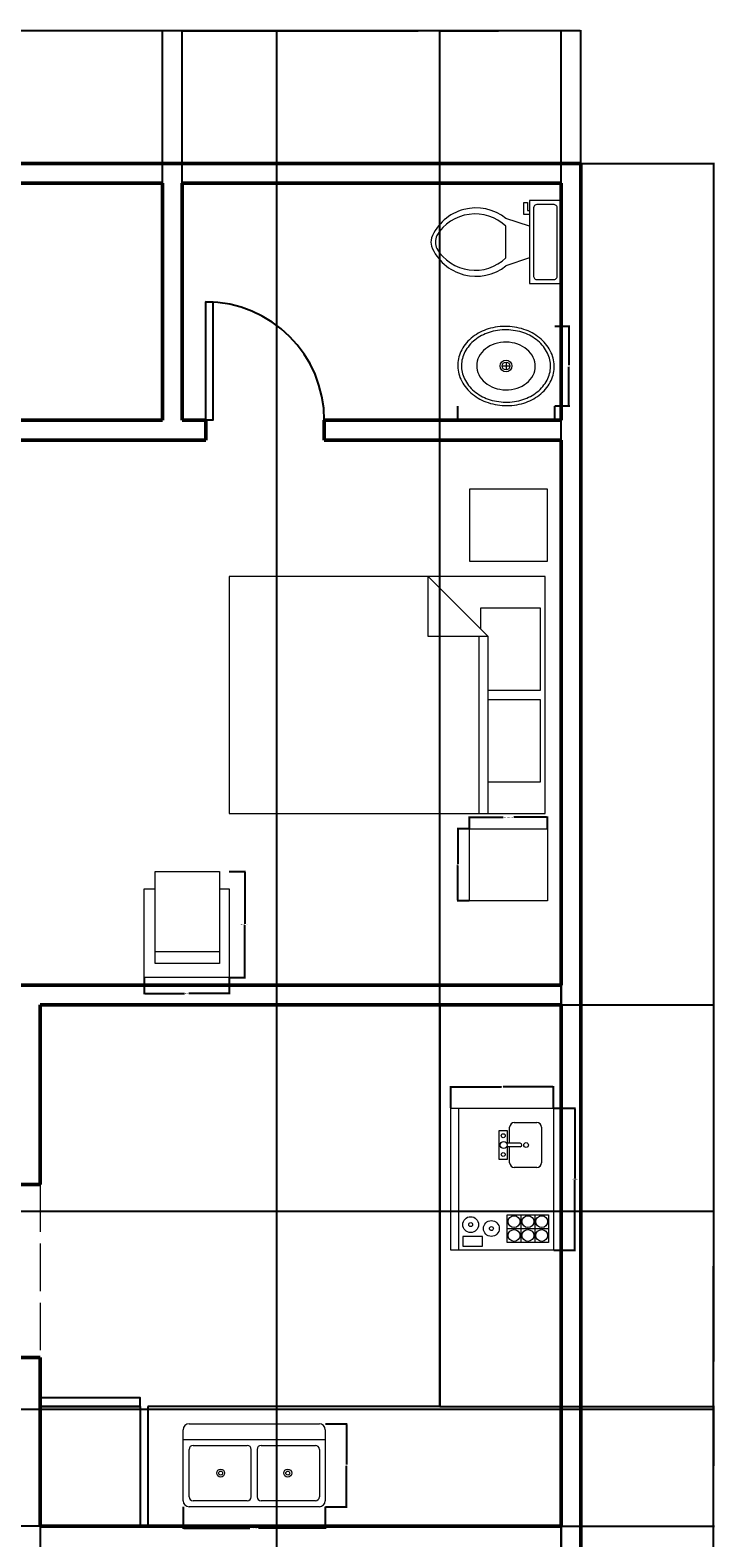
# Model space of a CAD drawing. Units: inches. Extents: x 115999 to 116502, y 188991 to 189729.
# Tile 5 of 5: x 116329 to 116502, y 189347 to 189729. Entities that reach past the tile are written whole.
import ezdxf

# ---------------------------------------------------------------- set-up
doc = ezdxf.new("R2010")
doc.units = ezdxf.units.IN
doc.linetypes.add('ACAD_ISO02W100', pattern=[15, 12, -3])
for name, color, linetype, lineweight in [('A-ANNO-DIMS', 2, 'Continuous', 18), ('A-DOOR', 4, 'Continuous', 25), ('A-FLOR-CASE', 9, 'Continuous', 25), ('A-FLOR-FIXT', 9, 'Continuous', 20), ('A-FURN', 8, 'Continuous', 18), ('A-WALL', 7, 'Continuous', 50), ('A-WALL-OVHD', 7, 'ACAD_ISO02W100', 18)]:
    doc.layers.add(name, color=color, linetype=linetype, lineweight=lineweight)
doc.styles.get("Standard").update_dxf_attribs({"font": 'arial.ttf'})
doc.dimstyles.get("Standard").update_dxf_attribs({"dimtxt": 0.18, "dimasz": 0.18, "dimexe": 0.18, "dimexo": 0.0625, "dimgap": 0.09, "dimtad": 0, "dimtih": 1, "dimtoh": 1, "dimdec": 4, "dimzin": 0, "dimdsep": 46, "dimtxsty": 'Standard', "dimcen": 0.09, "dimadec": 0, "dimazin": 0, "dimtfac": 1, "dimtdec": 4, "dimtofl": 0, "dimtmove": 0, "dimatfit": 3, "dimfxl": 1, "dimtolj": 1, "dimtzin": 0, "dimarcsym": 0})

# ---------------------------------------------------------------- blocks, each defined once
blk = doc.blocks.new('*U3')
for p, q in [((0, 0), (0, -5)), ((30, 0), (30, -5))]:
    blk.add_line(p, q)
blk.add_lwpolyline([(0, 0), (0, 30), (1.75, 30), (1.75, 0)], close=True)
blk.add_arc((0, 0), 30, 0, 90)
blk = doc.blocks.new('Wet Bar')
for p, q in [((0, 0), (36, 0)), ((0, -26), (0, 0)), ((36, 0), (36, -26)), ((0, -2), (36, -2)), ((3.5, -3), (1, -3)), ((1, -3), (1, -8)), ((3.5, -8), (3.5, -3)), ((1, -8), (3.5, -8)), ((2, -14.25), (9, -14.25)), ((2, -24.75), (2, -14.25)), ((5.5, -14.25), (5.5, -24.75)), ((9, -14.25), (9, -24.75)), ((26.2, -17.55), (26.2, -14.1284)), ((27.1001, -17.55), (27.1001, -14.1284)), ((2, -17.75), (9, -17.75)), ((9, -21.25), (2, -21.25)), ((36, -26), (0, -26)), ((9, -24.75), (2, -24.75))]:
    blk.add_line(p, q)
for points in [[(22.15, -14.85), (26.2, -14.85)], [(26.2, -14.25), (22.95, -14.25), (22.95, -12.2), (26.75, -12.2)], [(26.7487, -12.2), (30.3501, -12.2), (30.3501, -14.25), (27.1001, -14.25)], [(27.1001, -14.85), (31.15, -14.85)], [(20.95, -21.75), (20.95, -16.05)], [(32.3501, -16.05), (32.3501, -21.75)], [(31.15, -22.95), (22.15, -22.95)]]:
    blk.add_lwpolyline(points)
for centre, radius in [((6.5, -5), 2), ((6.5, -5), 0.5), ((5.5, -10.25), 2), ((5.5, -10.25), 0.5), ((3.75, -16), 1.5), ((7.25, -16), 1.5), ((24.25, -13.25), 0.5), ((26.65, -13.35), 0.9), ((29, -13.25), 0.5), ((3.75, -19.5), 1.5), ((7.25, -19.5), 1.5), ((26.65, -19.05), 0.6), ((3.75, -23), 1.5), ((7.25, -23), 1.5)]:
    blk.add_circle(centre, radius)
for centre, radius, start, end in [((22.2251, -16.125), 1.2772, 93.36646, 176.6335), ((31.075, -16.125), 1.2772, 3.366461, 86.63354), ((26.65, -17.55), 0.45, 180, 0), ((22.2251, -21.675), 1.2772, 183.3665, 266.6335), ((31.075, -21.675), 1.2772, 273.3665, 356.6335)]:
    blk.add_arc(centre, radius, start, end)
blk = doc.blocks.new('Sink-double - 36 in top')
for p, q in [((-18, -4), (18, -4)), ((-0.75, -18.5), (-0.75, -6.5)), ((0.75, -6.5), (0.75, -18.5))]:
    blk.add_line(p, q)
for points in [[(-16.5, 0), (16.5, 0)], [(-18, -19.5), (-18, -1.5)], [(18, -1.5), (18, -19.5)], [(-16.5, -18.5), (-16.5, -6.5)], [(-15.5, -5.5), (-1.75, -5.5)], [(1.75, -5.5), (15.5, -5.5)], [(16.5, -6.5), (16.5, -18.5)], [(16.5, -21), (-16.5, -21)], [(-1.75, -19.5), (-15.5, -19.5)], [(15.5, -19.5), (1.75, -19.5)]]:
    blk.add_lwpolyline(points)
for centre, radius in [((-8.5, -12.5), 1), ((-8.5, -12.5), 0.5), ((8.5, -12.5), 1), ((8.5, -12.5), 0.5)]:
    blk.add_circle(centre, radius)
for centre, radius, start, end in [((-16.5, -1.5), 1.5, 90, 180), ((16.5, -1.5), 1.5, 0, 90), ((-15.5, -6.5), 1, 90, 180), ((-1.75, -6.5), 1, 0, 90), ((1.75, -6.5), 1, 90, 180), ((15.5, -6.5), 1, 0, 90), ((-15.5, -18.5), 1, 180, 270), ((-1.75, -18.5), 1, 270, 0), ((1.75, -18.5), 1, 180, 270), ((15.5, -18.5), 1, 270, 0), ((-16.5, -19.5), 1.5, 180, 270), ((16.5, -19.5), 1.5, 270, 0)]:
    blk.add_arc(centre, radius, start, end)
blk = doc.blocks.new('Toilet - top')
for p, q in [((9.5, -6), (9.5, -2)), ((-10, -8.5), (-8, -8.5)), ((-10, -9.5), (-10, -8.5)), ((-7, -9.5), (-10, -9.5)), ((-8, -8.5), (-8, -8)), ((-7, -8), (-7, -9.5)), ((-4, -8), (-6, -14)), ((4, -8), (6, -14)), ((4, -14), (-4, -14))]:
    blk.add_line(p, q)
blk.add_lwpolyline([(10.5, -8), (10.5, 0), (-10.5, 0), (-10.5, -8)], close=True)
for points in [[(-9.5, -2), (-9.5, -6)], [(8.5, -1), (-8.5, -1)], [(-8.5, -7), (8.5, -7)]]:
    blk.add_lwpolyline(points)
for centre, radius, start, end in [((-8.62, -1.88), 0.884, 81.8699, 188.1301), ((8.62, -1.88), 0.884, 351.8699, 98.1301), ((-8.62, -6.12), 0.884, 171.8699, 278.1301), ((8.62, -6.12), 0.884, 261.8699, 8.1301), ((3.52, -21.58), 12.17, 141.4691, 247.9714), ((4.2, -21.82), 11.33, 136.3677, 238.9468), ((-3.52, -21.58), 12.17, 292.0284, 38.5307), ((-4.2, -21.82), 11.33, 301.053, 43.6321), ((0, -27.88), 4, 245.7318, 294.2682), ((0, -29), 4, 254.8605, 285.1395)]:
    blk.add_arc(centre, radius, start, end)
blk = doc.blocks.new('Sink - Oval top')
for p, q in [((-1, 0), (1, 0)), ((0, 1), (0, -1))]:
    blk.add_line(p, q)
for points in [[(-12.23, 0.39, 0.117634), (-11.46, -3.36, 0.104469), (-8.88, -6.8, 0.090016), (-5.08, -9.07, 0.08192), (-0.32, -10.02, 0.08192), (4.49, -9.38, 0.090016), (8.42, -7.36, 0.104469), (11.22, -4.09, 0.117634), (12.23, -0.39, 0.117634), (11.46, 3.36, 0.104469), (8.88, 6.8, 0.090016), (5.08, 9.07, 0.08192), (0.32, 10.02, 0.08192), (-4.49, 9.38, 0.090016), (-8.42, 7.36, 0.104469), (-11.22, 4.09, 0.117634)], [(-11.29, 0.16, 0.118622), (-10.52, -3.25, 0.104678), (-8.07, -6.36, 0.089562), (-4.54, -8.37, 0.081185), (-0.13, -9.15, 0.081185), (4.3, -8.49, 0.089562), (7.89, -6.58, 0.104678), (10.42, -3.55, 0.118622), (11.29, -0.16, 0.118622), (10.52, 3.25, 0.104678), (8.07, 6.36, 0.089562), (4.54, 8.37, 0.081185), (0.13, 9.15, 0.081185), (-4.3, 8.49, 0.089562), (-7.89, 6.58, 0.104678), (-10.42, 3.55, 0.118622)], [(-7.42, 0.08, 0.118283), (-6.91, -2.17, 0.104607), (-5.29, -4.21, 0.089718), (-2.97, -5.53, 0.081436), (-0.07, -6.04, 0.081436), (2.84, -5.59, 0.089718), (5.2, -4.33, 0.104607), (6.86, -2.32, 0.118283), (7.42, -0.08, 0.118283), (6.91, 2.17, 0.104607), (5.29, 4.21, 0.089718), (2.97, 5.53, 0.081436), (0.07, 6.04, 0.081436), (-2.84, 5.59, 0.089718), (-5.2, 4.33, 0.104607), (-6.86, 2.32, 0.118283)]]:
    blk.add_lwpolyline(points, format="xyb", close=True)
for radius in [1.5, 1]:
    blk.add_circle((0, 0), radius)
blk = doc.blocks.new('Bed - Queen')
for p, q in [((0, -80.00003), (0, 0)), ((0, 0), (59.99999, 0)), ((59.99999, 0), (59.99999, -80.00003)), ((7.99999, -1.2), (28.79998, -1.2)), ((7.99999, -14.4), (7.99999, -1.2)), ((28.79998, -1.2), (28.79998, -14.4)), ((31.19999, -1.2), (51.99999, -1.2)), ((31.19999, -14.4), (31.19999, -1.2)), ((51.99999, -1.2), (51.99999, -16.4)), ((0, -14.4), (44.8, -14.4)), ((59.99999, -29.6), (44.8, -14.4)), ((44.8, -14.4), (44.8, -29.6)), ((44.8, -16.8), (0, -16.8)), ((51.99999, -16.4), (46.79936, -16.4)), ((44.8, -29.6), (59.99999, -29.6)), ((59.99999, -80.00003), (0, -80.00003))]:
    blk.add_line(p, q)
blk = doc.blocks.new('CHAIR-ARM')
blk.add_line((2.71, 6.64), (19.06, 6.64))
blk.add_lwpolyline([(2.71, 26.84), (19.06, 26.84), (19.06, 3.59), (2.71, 3.59)], close=True)
blk.add_lwpolyline([(19.06, 22.51), (21.46, 22.51), (21.46, 0), (0, 0), (0, 22.51), (2.71, 22.51)])
blk = doc.blocks.new('TABLE-NIGHTSTAND')
blk.add_lwpolyline([(0, 18.2), (19.71, 18.2), (19.71, 0), (0, 0)], close=True)
blk = doc.blocks.new('*D17')
at = {"layer": 'A-ANNO-DIMS', "color": 0, "lineweight": -2, "transparency": 16777216}
for p, q in [((116439.84, 189526.56), (116439.84, 189529.63)), ((116440.02, 189529.45), (116448.32, 189529.45)), ((116459.37, 189529.45), (116451.07, 189529.45)), ((116459.55, 189526.56), (116459.55, 189529.63))]:
    blk.add_line(p, q, dxfattribs=at)
at = {"layer": 'A-ANNO-DIMS', "color": 0, "transparency": 16777216}
for points in [[(116440.02, 189529.48), (116440.02, 189529.42), (116439.84, 189529.45)], [(116459.37, 189529.48), (116459.37, 189529.42), (116459.55, 189529.45)]]:
    blk.add_solid(points, dxfattribs=at)
at = {"layer": 'Defpoints', "color": 0, "transparency": 16777216}
for p in [(116439.84, 189529.45), (116439.84, 189526.5), (116459.55, 189526.5)]:
    blk.add_point(p, dxfattribs=at)
at = {"layer": 'A-ANNO-DIMS', "color": 0, "transparency": 16777216, "insert": (116449.69, 189529.45), "char_height": 0.18, "attachment_point": 5}
blk.add_mtext('\\A1;NIGHTSTAND 20 TYP.', dxfattribs=at)
blk = doc.blocks.new('*D18')
at = {"layer": 'A-ANNO-DIMS', "color": 0, "lineweight": -2, "transparency": 16777216}
for p, q in [((116439.77, 189526.5), (116436.7, 189526.5)), ((116436.88, 189526.32), (116436.88, 189517.58)), ((116436.88, 189508.47), (116436.88, 189517.21)), ((116439.77, 189508.29), (116436.7, 189508.29))]:
    blk.add_line(p, q, dxfattribs=at)
at = {"layer": 'A-ANNO-DIMS', "color": 0, "transparency": 16777216}
for points in [[(116436.85, 189526.32), (116436.91, 189526.32), (116436.88, 189526.5)], [(116436.85, 189508.47), (116436.91, 189508.47), (116436.88, 189508.29)]]:
    blk.add_solid(points, dxfattribs=at)
at = {"layer": 'Defpoints', "color": 0, "transparency": 16777216}
for p in [(116439.84, 189526.5), (116436.88, 189508.29), (116439.84, 189508.29)]:
    blk.add_point(p, dxfattribs=at)
at = {"layer": 'A-ANNO-DIMS', "color": 0, "transparency": 16777216, "insert": (116436.88, 189517.39), "char_height": 0.18, "attachment_point": 5}
blk.add_mtext('\\A1;18 TYP.', dxfattribs=at)
blk = doc.blocks.new('*D23')
at = {"layer": 'A-ANNO-DIMS', "color": 0, "lineweight": -2, "transparency": 16777216}
for p, q in [((116436.8, 189633.57), (116436.8, 189629.77)), ((116461.35, 189633.57), (116461.35, 189629.77)), ((116436.98, 189629.95), (116448.14, 189629.95)), ((116461.17, 189629.95), (116450.01, 189629.95))]:
    blk.add_line(p, q, dxfattribs=at)
at = {"layer": 'A-ANNO-DIMS', "color": 0, "transparency": 16777216}
for points in [[(116436.98, 189629.98), (116436.98, 189629.92), (116436.8, 189629.95)], [(116461.17, 189629.98), (116461.17, 189629.92), (116461.35, 189629.95)]]:
    blk.add_solid(points, dxfattribs=at)
at = {"layer": 'Defpoints', "color": 0, "transparency": 16777216}
for p in [(116436.8, 189633.63), (116461.35, 189633.63), (116461.35, 189629.95)]:
    blk.add_point(p, dxfattribs=at)
at = {"layer": 'A-ANNO-DIMS', "color": 0, "transparency": 16777216, "insert": (116449.08, 189629.95), "char_height": 0.18, "attachment_point": 5}
blk.add_mtext('\\A1;BASIN 25 TYP.', dxfattribs=at)
blk = doc.blocks.new('*D24')
at = {"layer": 'A-ANNO-DIMS', "color": 0, "lineweight": -2, "transparency": 16777216}
for p, q in [((116461.41, 189653.77), (116465.21, 189653.77)), ((116465.03, 189653.59), (116465.03, 189643.88)), ((116465.03, 189633.81), (116465.03, 189643.52)), ((116461.41, 189633.63), (116465.21, 189633.63))]:
    blk.add_line(p, q, dxfattribs=at)
at = {"layer": 'A-ANNO-DIMS', "color": 0, "transparency": 16777216}
for points in [[(116465, 189653.59), (116465.06, 189653.59), (116465.03, 189653.77)], [(116465, 189633.81), (116465.06, 189633.81), (116465.03, 189633.63)]]:
    blk.add_solid(points, dxfattribs=at)
at = {"layer": 'Defpoints', "color": 0, "transparency": 16777216}
for p in [(116461.35, 189653.77), (116465.03, 189653.77), (116461.35, 189633.63)]:
    blk.add_point(p, dxfattribs=at)
at = {"layer": 'A-ANNO-DIMS', "color": 0, "transparency": 16777216, "insert": (116465.03, 189643.7), "char_height": 0.18, "attachment_point": 5}
blk.add_mtext('\\A1;20 TYP.', dxfattribs=at)
blk = doc.blocks.new('*D27')
at = {"layer": 'A-ANNO-DIMS', "color": 0, "lineweight": -2, "transparency": 16777216}
for p, q in [((116378.99, 189515.69), (116383.13, 189515.69)), ((116382.95, 189515.51), (116382.95, 189502.46)), ((116382.95, 189489.04), (116382.95, 189502.09)), ((116378.99, 189488.86), (116383.13, 189488.86))]:
    blk.add_line(p, q, dxfattribs=at)
at = {"layer": 'A-ANNO-DIMS', "color": 0, "transparency": 16777216}
for points in [[(116382.92, 189515.51), (116382.98, 189515.51), (116382.95, 189515.69)], [(116382.92, 189489.04), (116382.98, 189489.04), (116382.95, 189488.86)]]:
    blk.add_solid(points, dxfattribs=at)
at = {"layer": 'Defpoints', "color": 0, "transparency": 16777216}
for p in [(116378.93, 189515.69), (116382.95, 189515.69), (116378.93, 189488.86)]:
    blk.add_point(p, dxfattribs=at)
at = {"layer": 'A-ANNO-DIMS', "color": 0, "transparency": 16777216, "insert": (116382.95, 189502.28), "char_height": 0.18, "attachment_point": 5}
blk.add_mtext('\\A1;ARMCHAIR 27 TYP.', dxfattribs=at)
blk = doc.blocks.new('*D28')
at = {"layer": 'A-ANNO-DIMS', "color": 0, "lineweight": -2, "transparency": 16777216}
for p, q in [((116357.47, 189488.79), (116357.47, 189484.65)), ((116378.93, 189488.79), (116378.93, 189484.65)), ((116357.65, 189484.83), (116367.67, 189484.83)), ((116378.75, 189484.83), (116368.73, 189484.83))]:
    blk.add_line(p, q, dxfattribs=at)
at = {"layer": 'A-ANNO-DIMS', "color": 0, "transparency": 16777216}
for points in [[(116357.65, 189484.86), (116357.65, 189484.8), (116357.47, 189484.83)], [(116378.75, 189484.86), (116378.75, 189484.8), (116378.93, 189484.83)]]:
    blk.add_solid(points, dxfattribs=at)
at = {"layer": 'Defpoints', "color": 0, "transparency": 16777216}
for p in [(116357.47, 189488.86), (116378.93, 189488.86), (116378.93, 189484.83)]:
    blk.add_point(p, dxfattribs=at)
at = {"layer": 'A-ANNO-DIMS', "color": 0, "transparency": 16777216, "insert": (116368.2, 189484.83), "char_height": 0.18, "attachment_point": 5}
blk.add_mtext('\\A1;21 TYP.', dxfattribs=at)
blk = doc.blocks.new('*D29')
at = {"layer": 'A-ANNO-DIMS', "color": 0, "lineweight": -2, "transparency": 16777216}
for p, q in [((116461.19, 189455.82), (116466.71, 189455.82)), ((116466.53, 189455.64), (116466.53, 189438)), ((116466.53, 189420), (116466.53, 189437.64)), ((116461.19, 189419.82), (116466.71, 189419.82))]:
    blk.add_line(p, q, dxfattribs=at)
at = {"layer": 'A-ANNO-DIMS', "color": 0, "transparency": 16777216}
for points in [[(116466.5, 189455.64), (116466.56, 189455.64), (116466.53, 189455.82)], [(116466.5, 189420), (116466.56, 189420), (116466.53, 189419.82)]]:
    blk.add_solid(points, dxfattribs=at)
at = {"layer": 'Defpoints', "color": 0, "transparency": 16777216}
for p in [(116461.13, 189455.82), (116466.53, 189455.82), (116461.13, 189419.82)]:
    blk.add_point(p, dxfattribs=at)
at = {"layer": 'A-ANNO-DIMS', "color": 0, "transparency": 16777216, "insert": (116466.53, 189437.82), "char_height": 0.18, "attachment_point": 5}
blk.add_mtext('\\A1;WET BAR 36', dxfattribs=at)
blk = doc.blocks.new('*D30')
at = {"layer": 'A-ANNO-DIMS', "color": 0, "lineweight": -2, "transparency": 16777216}
for p, q in [((116435.13, 189455.88), (116435.13, 189461.4)), ((116435.31, 189461.22), (116447.91, 189461.22)), ((116460.95, 189461.22), (116448.35, 189461.22)), ((116461.13, 189455.88), (116461.13, 189461.4))]:
    blk.add_line(p, q, dxfattribs=at)
at = {"layer": 'A-ANNO-DIMS', "color": 0, "transparency": 16777216}
for points in [[(116435.31, 189461.25), (116435.31, 189461.19), (116435.13, 189461.22)], [(116460.95, 189461.25), (116460.95, 189461.19), (116461.13, 189461.22)]]:
    blk.add_solid(points, dxfattribs=at)
at = {"layer": 'Defpoints', "color": 0, "transparency": 16777216}
for p in [(116435.13, 189461.22), (116435.13, 189455.82), (116461.13, 189455.82)]:
    blk.add_point(p, dxfattribs=at)
at = {"layer": 'A-ANNO-DIMS', "color": 0, "transparency": 16777216, "insert": (116448.13, 189461.22), "char_height": 0.18, "attachment_point": 5}
blk.add_mtext('\\A1;26', dxfattribs=at)
blk = doc.blocks.new('*D31')
at = {"layer": 'A-ANNO-DIMS', "color": 0, "lineweight": -2, "transparency": 16777216}
for p, q in [((116367.31, 189354.84), (116367.31, 189349.32)), ((116403.31, 189354.84), (116403.31, 189349.32)), ((116367.49, 189349.5), (116384.21, 189349.5)), ((116403.13, 189349.5), (116386.4, 189349.5))]:
    blk.add_line(p, q, dxfattribs=at)
at = {"layer": 'A-ANNO-DIMS', "color": 0, "transparency": 16777216}
for points in [[(116367.49, 189349.53), (116367.49, 189349.47), (116367.31, 189349.5)], [(116403.13, 189349.53), (116403.13, 189349.47), (116403.31, 189349.5)]]:
    blk.add_solid(points, dxfattribs=at)
at = {"layer": 'Defpoints', "color": 0, "transparency": 16777216}
for p in [(116367.31, 189354.9), (116403.31, 189354.9), (116403.31, 189349.5)]:
    blk.add_point(p, dxfattribs=at)
at = {"layer": 'A-ANNO-DIMS', "color": 0, "transparency": 16777216, "insert": (116385.31, 189349.5), "char_height": 0.18, "attachment_point": 5}
blk.add_mtext('\\A1;DOUBLE SINK 36', dxfattribs=at)
blk = doc.blocks.new('*D32')
at = {"layer": 'A-ANNO-DIMS', "color": 0, "lineweight": -2, "transparency": 16777216}
for p, q in [((116403.37, 189375.9), (116408.89, 189375.9)), ((116408.71, 189375.72), (116408.71, 189365.58)), ((116408.71, 189355.08), (116408.71, 189365.22)), ((116403.37, 189354.9), (116408.89, 189354.9))]:
    blk.add_line(p, q, dxfattribs=at)
at = {"layer": 'A-ANNO-DIMS', "color": 0, "transparency": 16777216}
for points in [[(116408.68, 189375.72), (116408.74, 189375.72), (116408.71, 189375.9)], [(116408.68, 189355.08), (116408.74, 189355.08), (116408.71, 189354.9)]]:
    blk.add_solid(points, dxfattribs=at)
at = {"layer": 'Defpoints', "color": 0, "transparency": 16777216}
for p in [(116403.31, 189375.9), (116408.71, 189375.9), (116403.31, 189354.9)]:
    blk.add_point(p, dxfattribs=at)
at = {"layer": 'A-ANNO-DIMS', "color": 0, "transparency": 16777216, "insert": (116408.71, 189365.4), "char_height": 0.18, "attachment_point": 5}
blk.add_mtext('\\A1;21', dxfattribs=at)
blk = doc.blocks.new('*D33')
at = {"layer": 'A-ANNO-DIMS', "color": 0, "lineweight": -2, "transparency": 16777216}
for p, q in [((116088.06, 189088.01), (116088.06, 189728.73)), ((116088.24, 189728.55), (116277.77, 189728.55)), ((116467.88, 189728.55), (116278.35, 189728.55)), ((116468.06, 189088.01), (116468.06, 189728.73))]:
    blk.add_line(p, q, dxfattribs=at)
at = {"layer": 'A-ANNO-DIMS', "color": 0, "transparency": 16777216}
for points in [[(116088.24, 189728.58), (116088.24, 189728.52), (116088.06, 189728.55)], [(116467.88, 189728.58), (116467.88, 189728.52), (116468.06, 189728.55)]]:
    blk.add_solid(points, dxfattribs=at)
at = {"layer": 'Defpoints', "color": 0, "transparency": 16777216}
for p in [(116468.06, 189728.55), (116088.06, 189087.95), (116468.06, 189087.95)]:
    blk.add_point(p, dxfattribs=at)
at = {"layer": 'A-ANNO-DIMS', "color": 0, "transparency": 16777216, "insert": (116278.06, 189728.55), "char_height": 0.18, "attachment_point": 5}
blk.add_mtext('\\A1;380', dxfattribs=at)
blk = doc.blocks.new('*D34')
at = {"layer": 'A-ANNO-DIMS', "color": 0, "lineweight": -2, "transparency": 16777216}
for p, q in [((116468.13, 189694.95), (116501.84, 189694.95)), ((116501.66, 189694.77), (116501.66, 189391.63)), ((116501.66, 189088.13), (116501.66, 189391.27)), ((116468.13, 189087.95), (116501.84, 189087.95))]:
    blk.add_line(p, q, dxfattribs=at)
at = {"layer": 'A-ANNO-DIMS', "color": 0, "transparency": 16777216}
for points in [[(116501.63, 189694.77), (116501.69, 189694.77), (116501.66, 189694.95)], [(116501.63, 189088.13), (116501.69, 189088.13), (116501.66, 189087.95)]]:
    blk.add_solid(points, dxfattribs=at)
at = {"layer": 'Defpoints', "color": 0, "transparency": 16777216}
for p in [(116468.06, 189694.95), (116501.66, 189694.95), (116468.06, 189087.95)]:
    blk.add_point(p, dxfattribs=at)
at = {"layer": 'A-ANNO-DIMS', "color": 0, "transparency": 16777216, "insert": (116501.66, 189391.45), "char_height": 0.18, "attachment_point": 5}
blk.add_mtext('\\A1;607', dxfattribs=at)
blk = doc.blocks.new('*D36')
at = {"layer": 'A-ANNO-DIMS', "color": 0, "lineweight": -2, "transparency": 16777216}
for p, q in [((116194.06, 189690.01), (116194.06, 189728.73)), ((116194.24, 189728.55), (116277.78, 189728.55)), ((116361.88, 189728.55), (116278.34, 189728.55)), ((116362.06, 189690.01), (116362.06, 189728.73))]:
    blk.add_line(p, q, dxfattribs=at)
at = {"layer": 'A-ANNO-DIMS', "color": 0, "transparency": 16777216}
for points in [[(116194.24, 189728.58), (116194.24, 189728.52), (116194.06, 189728.55)], [(116361.88, 189728.58), (116361.88, 189728.52), (116362.06, 189728.55)]]:
    blk.add_solid(points, dxfattribs=at)
at = {"layer": 'Defpoints', "color": 0, "transparency": 16777216}
for p in [(116362.06, 189728.55), (116194.06, 189689.95), (116362.06, 189689.95)]:
    blk.add_point(p, dxfattribs=at)
at = {"layer": 'A-ANNO-DIMS', "color": 0, "transparency": 16777216, "insert": (116278.06, 189728.55), "char_height": 0.18, "attachment_point": 5}
blk.add_mtext('\\A1;168', dxfattribs=at)
blk = doc.blocks.new('*D37')
at = {"layer": 'A-ANNO-DIMS', "color": 0, "lineweight": -2, "transparency": 16777216}
for p, q in [((116367.06, 189690.01), (116367.06, 189728.73)), ((116367.24, 189728.55), (116414.84, 189728.55)), ((116462.88, 189728.55), (116415.28, 189728.55)), ((116463.06, 189690.01), (116463.06, 189728.73))]:
    blk.add_line(p, q, dxfattribs=at)
at = {"layer": 'A-ANNO-DIMS', "color": 0, "transparency": 16777216}
for points in [[(116367.24, 189728.58), (116367.24, 189728.52), (116367.06, 189728.55)], [(116462.88, 189728.58), (116462.88, 189728.52), (116463.06, 189728.55)]]:
    blk.add_solid(points, dxfattribs=at)
at = {"layer": 'Defpoints', "color": 0, "transparency": 16777216}
for p in [(116463.06, 189728.55), (116367.06, 189689.95), (116463.06, 189689.95)]:
    blk.add_point(p, dxfattribs=at)
at = {"layer": 'A-ANNO-DIMS', "color": 0, "transparency": 16777216, "insert": (116415.06, 189728.55), "char_height": 0.18, "attachment_point": 5}
blk.add_mtext('\\A1;96', dxfattribs=at)
blk = doc.blocks.new('*D44')
at = {"layer": 'A-ANNO-DIMS', "color": 0, "lineweight": -2, "transparency": 16777216}
for p, q in [((116277.06, 189624.88), (116277.06, 188991.26)), ((116463.06, 189624.88), (116463.06, 188991.26)), ((116277.24, 188991.44), (116369.78, 188991.44)), ((116462.88, 188991.44), (116370.34, 188991.44))]:
    blk.add_line(p, q, dxfattribs=at)
at = {"layer": 'A-ANNO-DIMS', "color": 0, "transparency": 16777216}
for points in [[(116277.24, 188991.47), (116277.24, 188991.41), (116277.06, 188991.44)], [(116462.88, 188991.47), (116462.88, 188991.41), (116463.06, 188991.44)]]:
    blk.add_solid(points, dxfattribs=at)
at = {"layer": 'Defpoints', "color": 0, "transparency": 16777216}
for p in [(116277.06, 189624.95), (116463.06, 189624.95), (116463.06, 188991.44)]:
    blk.add_point(p, dxfattribs=at)
at = {"layer": 'A-ANNO-DIMS', "color": 0, "transparency": 16777216, "insert": (116370.06, 188991.44), "char_height": 0.18, "attachment_point": 5}
blk.add_mtext('\\A1;186', dxfattribs=at)
blk = doc.blocks.new('*D49')
at = {"layer": 'A-ANNO-DIMS', "color": 0, "lineweight": -2, "transparency": 16777216}
for p, q in [((116331.06, 189349.88), (116331.06, 188991.26)), ((116463.06, 189349.88), (116463.06, 188991.26)), ((116331.24, 188991.44), (116396.78, 188991.44)), ((116462.88, 188991.44), (116397.34, 188991.44))]:
    blk.add_line(p, q, dxfattribs=at)
at = {"layer": 'A-ANNO-DIMS', "color": 0, "transparency": 16777216}
for points in [[(116331.24, 188991.47), (116331.24, 188991.41), (116331.06, 188991.44)], [(116462.88, 188991.47), (116462.88, 188991.41), (116463.06, 188991.44)]]:
    blk.add_solid(points, dxfattribs=at)
at = {"layer": 'Defpoints', "color": 0, "transparency": 16777216}
for p in [(116331.06, 189349.95), (116463.06, 189349.95), (116463.06, 188991.44)]:
    blk.add_point(p, dxfattribs=at)
at = {"layer": 'A-ANNO-DIMS', "color": 0, "transparency": 16777216, "insert": (116397.06, 188991.44), "char_height": 0.18, "attachment_point": 5}
blk.add_mtext('\\A1;132', dxfattribs=at)
blk = doc.blocks.new('*D52')
at = {"layer": 'A-ANNO-DIMS', "color": 0, "lineweight": -2, "transparency": 16777216}
for p, q in [((116463.13, 189481.95), (116501.84, 189481.95)), ((116501.66, 189481.77), (116501.66, 189416.13)), ((116501.66, 189350.13), (116501.66, 189415.76)), ((116463.13, 189349.95), (116501.84, 189349.95))]:
    blk.add_line(p, q, dxfattribs=at)
at = {"layer": 'A-ANNO-DIMS', "color": 0, "transparency": 16777216}
for points in [[(116501.63, 189481.77), (116501.69, 189481.77), (116501.66, 189481.95)], [(116501.63, 189350.13), (116501.69, 189350.13), (116501.66, 189349.95)]]:
    blk.add_solid(points, dxfattribs=at)
at = {"layer": 'Defpoints', "color": 0, "transparency": 16777216}
for p in [(116463.06, 189481.95), (116501.66, 189481.95), (116463.06, 189349.95)]:
    blk.add_point(p, dxfattribs=at)
at = {"layer": 'A-ANNO-DIMS', "color": 0, "transparency": 16777216, "insert": (116501.66, 189415.95), "char_height": 0.18, "attachment_point": 5}
blk.add_mtext('\\A1;132', dxfattribs=at)
blk = doc.blocks.new('*D53')
at = {"layer": 'A-ANNO-DIMS', "color": 0, "lineweight": -2, "transparency": 16777216}
for p, q in [((116331, 189436.5), (115999.04, 189436.5)), ((115999.22, 189436.32), (115999.22, 189414.77)), ((115999.22, 189392.85), (115999.22, 189414.41)), ((116331, 189392.67), (115999.04, 189392.67))]:
    blk.add_line(p, q, dxfattribs=at)
at = {"layer": 'A-ANNO-DIMS', "color": 0, "transparency": 16777216}
for points in [[(115999.19, 189436.32), (115999.25, 189436.32), (115999.22, 189436.5)], [(115999.19, 189392.85), (115999.25, 189392.85), (115999.22, 189392.67)]]:
    blk.add_solid(points, dxfattribs=at)
at = {"layer": 'Defpoints', "color": 0, "transparency": 16777216}
for p in [(115999.22, 189436.5), (116331.06, 189436.5), (116331.06, 189392.67)]:
    blk.add_point(p, dxfattribs=at)
at = {"layer": 'A-ANNO-DIMS', "color": 0, "transparency": 16777216, "insert": (115999.22, 189414.59), "char_height": 0.18, "attachment_point": 5}
blk.add_mtext('\\A1;43.83', dxfattribs=at)
blk = doc.blocks.new('*D65')
at = {"layer": 'A-ANNO-DIMS', "color": 0, "lineweight": -2, "transparency": 16777216}
for p, q in [((116391.06, 189309.01), (116391.06, 189728.73)), ((116391.24, 189728.55), (116426.85, 189728.55)), ((116462.88, 189728.55), (116427.28, 189728.55)), ((116463.06, 189237.01), (116463.06, 189728.73))]:
    blk.add_line(p, q, dxfattribs=at)
at = {"layer": 'A-ANNO-DIMS', "color": 0, "transparency": 16777216}
for points in [[(116391.24, 189728.58), (116391.24, 189728.52), (116391.06, 189728.55)], [(116462.88, 189728.58), (116462.88, 189728.52), (116463.06, 189728.55)]]:
    blk.add_solid(points, dxfattribs=at)
at = {"layer": 'Defpoints', "color": 0, "transparency": 16777216}
for p in [(116463.06, 189728.55), (116391.06, 189308.95), (116463.06, 189236.95)]:
    blk.add_point(p, dxfattribs=at)
at = {"layer": 'A-ANNO-DIMS', "color": 0, "transparency": 16777216, "insert": (116427.06, 189728.55), "char_height": 0.18, "attachment_point": 5}
blk.add_mtext('\\A1;72', dxfattribs=at)
blk = doc.blocks.new('*D67')
at = {"layer": 'A-ANNO-DIMS', "color": 0, "lineweight": -2, "transparency": 16777216}
for p, q in [((116331, 189392.67), (115999.04, 189392.67)), ((115999.22, 189392.49), (115999.22, 189371.49)), ((115999.22, 189350.13), (115999.22, 189371.13)), ((116331, 189349.95), (115999.04, 189349.95))]:
    blk.add_line(p, q, dxfattribs=at)
at = {"layer": 'A-ANNO-DIMS', "color": 0, "transparency": 16777216}
for points in [[(115999.19, 189392.49), (115999.25, 189392.49), (115999.22, 189392.67)], [(115999.19, 189350.13), (115999.25, 189350.13), (115999.22, 189349.95)]]:
    blk.add_solid(points, dxfattribs=at)
at = {"layer": 'Defpoints', "color": 0, "transparency": 16777216}
for p in [(115999.22, 189392.67), (116331.06, 189392.67), (116331.06, 189349.95)]:
    blk.add_point(p, dxfattribs=at)
at = {"layer": 'A-ANNO-DIMS', "color": 0, "transparency": 16777216, "insert": (115999.22, 189371.31), "char_height": 0.18, "attachment_point": 5}
blk.add_mtext('\\A1;42.73', dxfattribs=at)
blk = doc.blocks.new('*D68')
at = {"layer": 'A-ANNO-DIMS', "color": 0, "lineweight": -2, "transparency": 16777216}
for p, q in [((116432.28, 189380.32), (116432.28, 189728.73)), ((116432.46, 189728.55), (116447.21, 189728.55)), ((116462.88, 189728.55), (116448.13, 189728.55)), ((116463.06, 189350.01), (116463.06, 189728.73))]:
    blk.add_line(p, q, dxfattribs=at)
at = {"layer": 'A-ANNO-DIMS', "color": 0, "transparency": 16777216}
for points in [[(116432.46, 189728.58), (116432.46, 189728.52), (116432.28, 189728.55)], [(116462.88, 189728.58), (116462.88, 189728.52), (116463.06, 189728.55)]]:
    blk.add_solid(points, dxfattribs=at)
at = {"layer": 'Defpoints', "color": 0, "transparency": 16777216}
for p in [(116463.06, 189728.55), (116432.28, 189380.26), (116463.06, 189349.95)]:
    blk.add_point(p, dxfattribs=at)
at = {"layer": 'A-ANNO-DIMS', "color": 0, "transparency": 16777216, "insert": (116447.67, 189728.55), "char_height": 0.18, "attachment_point": 5}
blk.add_mtext('\\A1;30.785', dxfattribs=at)
blk = doc.blocks.new('*D69')
at = {"layer": 'A-ANNO-DIMS', "color": 0, "lineweight": -2, "transparency": 16777216}
for p, q in [((116432.34, 189380.26), (116501.84, 189380.26)), ((116501.66, 189380.08), (116501.66, 189365.28)), ((116501.66, 189350.13), (116501.66, 189364.92)), ((116463.13, 189349.95), (116501.84, 189349.95))]:
    blk.add_line(p, q, dxfattribs=at)
at = {"layer": 'A-ANNO-DIMS', "color": 0, "transparency": 16777216}
for points in [[(116501.63, 189380.08), (116501.69, 189380.08), (116501.66, 189380.26)], [(116501.63, 189350.13), (116501.69, 189350.13), (116501.66, 189349.95)]]:
    blk.add_solid(points, dxfattribs=at)
at = {"layer": 'Defpoints', "color": 0, "transparency": 16777216}
for p in [(116432.28, 189380.26), (116463.06, 189349.95), (116501.66, 189349.95)]:
    blk.add_point(p, dxfattribs=at)
at = {"layer": 'A-ANNO-DIMS', "color": 0, "transparency": 16777216, "insert": (116501.66, 189365.1), "char_height": 0.18, "attachment_point": 5}
blk.add_mtext('\\A1;30.31', dxfattribs=at)
blk = doc.blocks.new('*D79')
at = {"layer": 'A-ANNO-DIMS', "color": 0, "lineweight": -2, "transparency": 16777216}
for p, q in [((116221.53, 189429.68), (116501.84, 189429.68)), ((116501.66, 189429.5), (116501.66, 189404.83)), ((116501.66, 189379.81), (116501.66, 189404.47)), ((116221.53, 189379.63), (116501.84, 189379.63))]:
    blk.add_line(p, q, dxfattribs=at)
at = {"layer": 'A-ANNO-DIMS', "color": 0, "transparency": 16777216}
for points in [[(116501.63, 189429.5), (116501.69, 189429.5), (116501.66, 189429.68)], [(116501.63, 189379.81), (116501.69, 189379.81), (116501.66, 189379.63)]]:
    blk.add_solid(points, dxfattribs=at)
at = {"layer": 'Defpoints', "color": 0, "transparency": 16777216}
for p in [(116221.47, 189429.68), (116501.66, 189429.68), (116221.47, 189379.63)]:
    blk.add_point(p, dxfattribs=at)
at = {"layer": 'A-ANNO-DIMS', "color": 0, "transparency": 16777216, "insert": (116501.66, 189404.65), "char_height": 0.18, "attachment_point": 5}
blk.add_mtext('\\A1;50.05', dxfattribs=at)

msp = doc.modelspace()

# ---------------------------------------------------------------- linework, layer by layer
at = {"layer": 'A-FLOR-CASE'}
for p, q in [((116432.2777, 189481.9469), (116432.2777, 189380.2568)), ((116356.3868, 189380.2568), (116331.0631, 189380.2568)), ((116356.3868, 189380.2568), (116356.3868, 189349.9469)), ((116432.2777, 189380.2568), (116358.3868, 189380.2568)), ((116358.3868, 189380.2568), (116358.3868, 189349.9469))]:
    msp.add_line(p, q, dxfattribs=at)
msp.add_lwpolyline([(116331.0631, 189380.2568), (116356.3868, 189380.2568), (116356.3868, 189382.454), (116331.0631, 189382.454)], close=True, dxfattribs=at)
at = {"layer": 'A-WALL'}
for p, q in [((116088.0631, 189694.9469), (116468.0631, 189694.9469)), ((116468.0631, 189694.9469), (116468.0631, 189087.9469)), ((116194.0631, 189689.9469), (116362.0631, 189689.9469)), ((116362.0631, 189689.9469), (116362.0631, 189629.9469)), ((116367.0631, 189689.9469), (116367.0631, 189629.9469)), ((116367.0631, 189689.9469), (116463.0631, 189689.9469)), ((116463.0631, 189689.9469), (116463.0631, 189629.9469)), ((116313.0631, 189629.9469), (116362.0631, 189629.9469)), ((116367.0631, 189629.9469), (116373.0631, 189629.9469)), ((116373.0631, 189629.9469), (116373.0631, 189624.9469)), ((116403.0631, 189629.9469), (116403.0631, 189624.9469)), ((116403.0631, 189629.9469), (116463.0631, 189629.9469)), ((116313.0631, 189624.9469), (116373.0631, 189624.9469)), ((116403.0631, 189624.9469), (116463.0631, 189624.9469)), ((116463.0631, 189624.9469), (116463.0631, 189486.9469)), ((116325.0631, 189486.9469), (116463.0631, 189486.9469)), ((116331.0631, 189481.9469), (116331.0631, 189436.5016)), ((116331.0631, 189481.9469), (116463.0631, 189481.9469)), ((116463.0631, 189481.9469), (116463.0631, 189349.9469)), ((116326.0631, 189436.5016), (116331.0631, 189436.5016)), ((116326.0631, 189392.6745), (116331.0631, 189392.6745)), ((116331.0631, 189392.6745), (116331.0631, 189349.9469)), ((116331.0631, 189349.9469), (116463.0631, 189349.9469))]:
    msp.add_line(p, q, dxfattribs=at)
at = {"layer": 'A-WALL-OVHD'}
msp.add_line((116331.0631, 189436.5016), (116331.0631, 189392.6745), dxfattribs=at)

# ---------------------------------------------------------------- block references
at = {"layer": 'A-DOOR'}
msp.add_blockref('*U3', (116373.0631, 189629.9469), dxfattribs=at)
at = {"layer": 'A-FLOR-FIXT'}
for name, p, rotation in [('Toilet - top', (116463.0631, 189675.0657), 270), ('Wet Bar', (116435.128, 189419.8211), 90)]:
    msp.add_blockref(name, p, dxfattribs=dict(at, rotation=rotation))
for name, p in [('Sink - Oval top', (116449.0766, 189643.6992)), ('Sink-double - 36 in top', (116385.308, 189375.9002))]:
    msp.add_blockref(name, p, dxfattribs=at)
at = {"layer": 'A-FURN', "extrusion": (0, 0, -1), "zscale": -1}
msp.add_blockref('TABLE-NIGHTSTAND', (-116459.5459, 189594.2971), dxfattribs=at)
at = {"layer": 'A-FURN', "xscale": -1, "rotation": 270}
msp.add_blockref('Bed - Queen', (116458.9841, 189530.3971), dxfattribs=at)
at = {"layer": 'A-FURN', "rotation": 180}
msp.add_blockref('TABLE-NIGHTSTAND', (116459.5459, 189526.497), dxfattribs=at)
at = {"layer": 'A-FURN'}
msp.add_blockref('CHAIR-ARM', (116357.4742, 189488.8569), dxfattribs=at)

# ---------------------------------------------------------------- dimensions: what is measured, and where the dimension line sits
at = {"layer": 'A-ANNO-DIMS'}
for base, p1, p2, override, picture, middle in [((116468.0631, 189728.5469), (116088.0631, 189087.9469), (116468.0631, 189087.9469), {"dimdec": 0, "dimlfac": 1, "dimrnd": 0, "dimzin": 0, "dimdsep": 46, "dimlunit": 2}, '*D33', (116278.0631, 189728.5469)), ((116362.0631, 189728.5469), (116194.0631, 189689.9469), (116362.0631, 189689.9469), {"dimdec": 0, "dimlfac": 1, "dimrnd": 0, "dimzin": 0, "dimdsep": 46, "dimlunit": 2}, '*D36', (116278.0631, 189728.5469)), ((116463.0631, 189728.5469), (116367.0631, 189689.9469), (116463.0631, 189689.9469), {"dimdec": 0, "dimlfac": 1, "dimrnd": 0, "dimzin": 0, "dimdsep": 46, "dimlunit": 2}, '*D37', (116415.0631, 189728.5469)), ((116463.0631, 189728.5469), (116391.0631, 189308.9469), (116463.0631, 189236.9469), {"dimdec": 0, "dimlfac": 1, "dimrnd": 0, "dimzin": 0, "dimdsep": 46, "dimlunit": 2}, '*D65', (116427.0631, 189728.5469)), ((116463.0631, 189728.5469), (116432.2777, 189380.2568), (116463.0631, 189349.9469), {"dimdec": 3, "dimlfac": 1, "dimrnd": 0, "dimzin": 0, "dimdsep": 46, "dimlunit": 2}, '*D68', (116447.6704, 189728.5469)), ((116463.0631, 188991.4393), (116277.0631, 189624.9469), (116463.0631, 189624.9469), {"dimdec": 0, "dimlfac": 1, "dimrnd": 0, "dimzin": 0, "dimdsep": 46, "dimlunit": 2}, '*D44', (116370.0631, 188991.4393)), ((116463.0631, 188991.4393), (116331.0631, 189349.9469), (116463.0631, 189349.9469), {"dimdec": 0, "dimlfac": 1, "dimrnd": 0, "dimzin": 0, "dimdsep": 46, "dimlunit": 2}, '*D49', (116397.0631, 188991.4393))]:
    dim = msp.add_linear_dim(base=base, p1=p1, p2=p2, dimstyle='Standard', override=override, dxfattribs=at)
    dim.commit()
    dim.dimension.update_dxf_attribs({"geometry": picture, "text_midpoint": middle})
for base, p1, p2, angle, override, picture, middle in [((116501.6631, 189694.9469), (116468.0631, 189087.9469), (116468.0631, 189694.9469), 90, {"dimdec": 0, "dimlfac": 1, "dimrnd": 0, "dimzin": 0, "dimdsep": 46, "dimlunit": 2}, '*D34', (116501.6631, 189391.4469)), ((116501.6631, 189481.9469), (116463.0631, 189349.9469), (116463.0631, 189481.9469), 90, {"dimdec": 0, "dimlfac": 1, "dimrnd": 0, "dimzin": 0, "dimdsep": 46, "dimlunit": 2}, '*D52', (116501.6631, 189415.9469)), ((116435.128, 189461.2211), (116461.128, 189455.8211), (116435.128, 189455.8211), 180, {"dimdec": 0, "dimlfac": 1, "dimrnd": 0, "dimzin": 0, "dimdsep": 46, "dimlunit": 2}, '*D30', (116448.128, 189461.2211)), ((115999.2211, 189436.5016), (116331.0631, 189392.6745), (116331.0631, 189436.5016), 90, {"dimdec": 2, "dimlfac": 1, "dimrnd": 0, "dimzin": 0, "dimdsep": 46, "dimlunit": 2}, '*D53', (115999.2211, 189414.588)), ((116501.6631, 189429.6768), (116221.4703, 189379.6257), (116221.4703, 189429.6768), 90, {"dimdec": 2, "dimlfac": 1, "dimrnd": 0, "dimzin": 0, "dimdsep": 46, "dimlunit": 2}, '*D79', (116501.6631, 189404.6513)), ((115999.2211, 189392.6745), (116331.0631, 189349.9469), (116331.0631, 189392.6745), 90, {"dimdec": 2, "dimlfac": 1, "dimrnd": 0, "dimzin": 0, "dimdsep": 46, "dimlunit": 2}, '*D67', (115999.2211, 189371.3107)), ((116501.6631, 189349.9469), (116432.2777, 189380.2568), (116463.0631, 189349.9469), 90, {"dimdec": 2, "dimlfac": 1, "dimrnd": 0, "dimzin": 0, "dimdsep": 46, "dimlunit": 2}, '*D69', (116501.6631, 189365.1019)), ((116408.708, 189375.9002), (116403.308, 189354.9002), (116403.308, 189375.9002), 90, {"dimdec": 0, "dimlfac": 1, "dimrnd": 0, "dimzin": 0, "dimdsep": 46, "dimlunit": 2}, '*D32', (116408.708, 189365.4002))]:
    dim = msp.add_linear_dim(base=base, p1=p1, p2=p2, angle=angle, dimstyle='Standard', override=override, dxfattribs=at)
    dim.commit()
    dim.dimension.update_dxf_attribs({"geometry": picture, "text_midpoint": middle})
for base, p1, p2, angle, text, picture, middle in [((116465.0347, 189653.7675), (116461.352, 189633.6309), (116461.352, 189653.7675), 90, '<> TYP.', '*D24', (116465.0347, 189643.6992)), ((116439.836, 189529.4535), (116459.5459, 189526.497), (116439.836, 189526.497), 180, 'NIGHTSTAND <> TYP.', '*D17', (116449.6909, 189529.4535)), ((116436.8795, 189508.2926), (116439.836, 189526.497), (116439.836, 189508.2926), 270, '<> TYP.', '*D18', (116436.8795, 189517.3948)), ((116382.9546, 189515.6932), (116378.9292, 189488.8569), (116378.9292, 189515.6932), 90, 'ARMCHAIR <> TYP.', '*D27', (116382.9546, 189502.275)), ((116466.528, 189455.8211), (116461.128, 189419.8211), (116461.128, 189455.8211), 90, 'WET BAR <>', '*D29', (116466.528, 189437.8211))]:
    dim = msp.add_linear_dim(base=base, p1=p1, p2=p2, angle=angle, text=text, dimstyle='Standard', override={"dimdec": 0, "dimlfac": 1, "dimrnd": 0, "dimzin": 0, "dimdsep": 46, "dimlunit": 2}, dxfattribs=at)
    dim.commit()
    dim.dimension.update_dxf_attribs({"geometry": picture, "text_midpoint": middle})
for base, p1, p2, text, picture, middle in [((116461.352, 189629.9483), (116436.8011, 189633.6309), (116461.352, 189633.6309), 'BASIN <> TYP.', '*D23', (116449.0766, 189629.9483)), ((116378.9292, 189484.8315), (116357.4742, 189488.8569), (116378.9292, 189488.8569), '<> TYP.', '*D28', (116368.2017, 189484.8315)), ((116403.308, 189349.5002), (116367.308, 189354.9002), (116403.308, 189354.9002), 'DOUBLE SINK <>', '*D31', (116385.308, 189349.5002))]:
    dim = msp.add_linear_dim(base=base, p1=p1, p2=p2, text=text, dimstyle='Standard', override={"dimdec": 0, "dimlfac": 1, "dimrnd": 0, "dimzin": 0, "dimdsep": 46, "dimlunit": 2}, dxfattribs=at)
    dim.commit()
    dim.dimension.update_dxf_attribs({"geometry": picture, "text_midpoint": middle})

doc.saveas('drawing.dxf')
